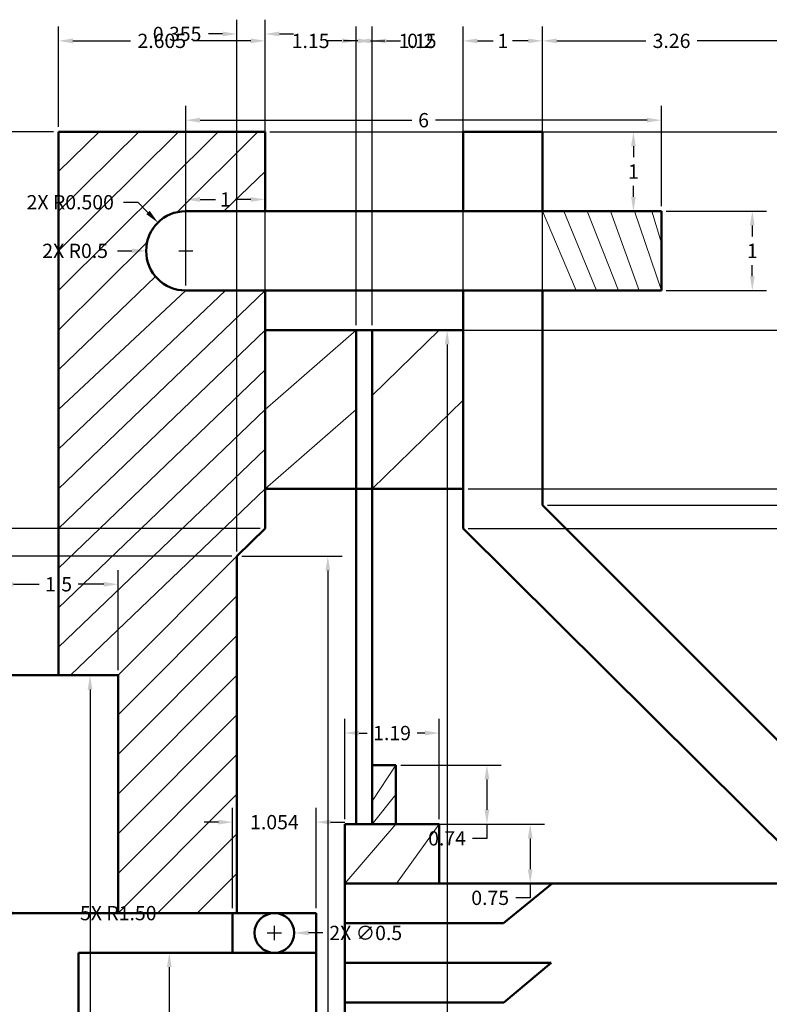
# Model space of a CAD drawing. Units: inches. Extents: x 15.4 to 41.1, y -0.4 to 25.1.
# Tile 3 of 4: x 20.3 to 29.7, y 12.7 to 25.1. Entities that reach past the tile are written whole.
import ezdxf

# ---------------------------------------------------------------- set-up
doc = ezdxf.new("R2010")
doc.units = ezdxf.units.IN
doc.header["$MEASUREMENT"] = 0
for name, color, linetype, lineweight in [('M-DIMS', 2, 'Continuous', 18), ('M-HATC', 8, 'Continuous', 18), ('M-OUTL', 7, 'Continuous', 50)]:
    doc.layers.add(name, color=color, linetype=linetype, lineweight=lineweight)
doc.styles.get("Standard").update_dxf_attribs({"font": 'arial.ttf'})
doc.dimstyles.get("Standard").update_dxf_attribs({"dimtxt": 0.18, "dimasz": 0.18, "dimexe": 0.18, "dimexo": 0.0625, "dimgap": 0.09, "dimtad": 0, "dimtih": 1, "dimtoh": 1, "dimdec": 4, "dimzin": 0, "dimdsep": 46, "dimtxsty": 'Standard', "dimcen": 0.09, "dimadec": 0, "dimazin": 0, "dimtfac": 1, "dimtdec": 4, "dimtofl": 0, "dimtmove": 0, "dimatfit": 3, "dimfxl": 1, "dimtolj": 1, "dimtzin": 0, "dimarcsym": 0})

# ---------------------------------------------------------------- blocks, each defined once
blk = doc.blocks.new('*D2')
at = {"layer": 'Defpoints', "color": 0, "transparency": 16777216}
for p in [(16.366, 23.727), (20.763, 23.727), (20.763, 1.022)]:
    blk.add_point(p, dxfattribs=at)
at = {"layer": 'M-DIMS', "color": 0, "lineweight": -2, "transparency": 16777216}
for p, q in [((20.7, 23.727), (16.186, 23.727)), ((16.366, 23.547), (16.366, 12.557)), ((16.366, 1.202), (16.366, 12.193)), ((20.7, 1.022), (16.186, 1.022))]:
    blk.add_line(p, q, dxfattribs=at)
at = {"layer": 'M-DIMS', "color": 0, "transparency": 16777216}
for points in [[(16.336, 23.547), (16.396, 23.547), (16.366, 23.727)], [(16.336, 1.202), (16.396, 1.202), (16.366, 1.022)]]:
    blk.add_solid(points, dxfattribs=at)
at = {"layer": 'M-DIMS', "color": 0, "transparency": 16777216, "insert": (16.366, 12.375), "char_height": 0.18, "attachment_point": 5}
blk.add_mtext('\\A1;22.705', dxfattribs=at)
blk = doc.blocks.new('*D3')
at = {"layer": 'Defpoints', "color": 0, "transparency": 16777216}
for p in [(23.368, 24.875), (20.763, 23.727), (23.368, 23.727)]:
    blk.add_point(p, dxfattribs=at)
at = {"layer": 'M-DIMS', "color": 0, "lineweight": -2, "transparency": 16777216}
for p, q in [((20.763, 23.79), (20.763, 25.055)), ((23.368, 23.79), (23.368, 25.055)), ((20.943, 24.875), (21.669, 24.875)), ((23.188, 24.875), (22.461, 24.875))]:
    blk.add_line(p, q, dxfattribs=at)
at = {"layer": 'M-DIMS', "color": 0, "transparency": 16777216}
for points in [[(20.943, 24.905), (20.943, 24.845), (20.763, 24.875)], [(23.188, 24.905), (23.188, 24.845), (23.368, 24.875)]]:
    blk.add_solid(points, dxfattribs=at)
at = {"layer": 'M-DIMS', "color": 0, "transparency": 16777216, "insert": (22.065, 24.875), "char_height": 0.18, "attachment_point": 5}
blk.add_mtext('\\A1;2.605', dxfattribs=at)
blk = doc.blocks.new('*D4')
at = {"layer": 'Defpoints', "color": 0, "transparency": 16777216}
for p in [(24.51758, 24.874511), (23.36758, 21.227011), (24.51758, 21.227011)]:
    blk.add_point(p, dxfattribs=at)
at = {"layer": 'M-DIMS', "color": 0, "lineweight": -2, "transparency": 16777216}
for p, q in [((23.36758, 21.289511), (23.36758, 25.054511)), ((24.51758, 21.289511), (24.51758, 25.054511)), ((23.18758, 24.874511), (23.00758, 24.874511)), ((24.69758, 24.874511), (24.87758, 24.874511))]:
    blk.add_line(p, q, dxfattribs=at)
at = {"layer": 'M-DIMS', "color": 0, "transparency": 16777216}
for points in [[(23.18758, 24.904511), (23.18758, 24.844511), (23.36758, 24.874511)], [(24.69758, 24.904511), (24.69758, 24.844511), (24.51758, 24.874511)]]:
    blk.add_solid(points, dxfattribs=at)
at = {"layer": 'M-DIMS', "color": 0, "transparency": 16777216, "insert": (23.94258, 24.874511), "char_height": 0.18, "attachment_point": 5}
blk.add_mtext('\\A1;1.15', dxfattribs=at)
blk = doc.blocks.new('*D5')
at = {"layer": 'Defpoints', "color": 0, "transparency": 16777216}
for p in [(24.718, 24.875), (24.518, 21.227), (24.718, 21.227)]:
    blk.add_point(p, dxfattribs=at)
at = {"layer": 'M-DIMS', "color": 0, "lineweight": -2, "transparency": 16777216}
for p, q in [((24.518, 21.29), (24.518, 25.055)), ((24.718, 21.29), (24.718, 25.055)), ((24.338, 24.875), (24.158, 24.875)), ((24.898, 24.875), (25.078, 24.875))]:
    blk.add_line(p, q, dxfattribs=at)
at = {"layer": 'M-DIMS', "color": 0, "transparency": 16777216}
for points in [[(24.338, 24.905), (24.338, 24.845), (24.518, 24.875)], [(24.898, 24.905), (24.898, 24.845), (24.718, 24.875)]]:
    blk.add_solid(points, dxfattribs=at)
at = {"layer": 'M-DIMS', "color": 0, "transparency": 16777216, "insert": (25.331, 24.875), "char_height": 0.18, "attachment_point": 5}
blk.add_mtext('\\A1;0.2', dxfattribs=at)
blk = doc.blocks.new('*D6')
at = {"layer": 'Defpoints', "color": 0, "transparency": 16777216}
for p in [(25.86758, 24.874511), (24.71758, 21.227011), (25.86758, 21.227011)]:
    blk.add_point(p, dxfattribs=at)
at = {"layer": 'M-DIMS', "color": 0, "lineweight": -2, "transparency": 16777216}
for p, q in [((24.71758, 21.289511), (24.71758, 25.054511)), ((25.86758, 21.289511), (25.86758, 25.054511)), ((24.53758, 24.874511), (24.35758, 24.874511)), ((26.04758, 24.874511), (26.22758, 24.874511))]:
    blk.add_line(p, q, dxfattribs=at)
at = {"layer": 'M-DIMS', "color": 0, "transparency": 16777216}
for points in [[(24.53758, 24.904511), (24.53758, 24.844511), (24.71758, 24.874511)], [(26.04758, 24.904511), (26.04758, 24.844511), (25.86758, 24.874511)]]:
    blk.add_solid(points, dxfattribs=at)
at = {"layer": 'M-DIMS', "color": 0, "transparency": 16777216, "insert": (25.29258, 24.874511), "char_height": 0.18, "attachment_point": 5}
blk.add_mtext('\\A1;1.15', dxfattribs=at)
blk = doc.blocks.new('*D7')
at = {"layer": 'Defpoints', "color": 0, "transparency": 16777216}
for p in [(26.868, 24.875), (25.868, 23.727), (26.868, 23.727)]:
    blk.add_point(p, dxfattribs=at)
at = {"layer": 'M-DIMS', "color": 0, "lineweight": -2, "transparency": 16777216}
for p, q in [((25.868, 23.79), (25.868, 25.055)), ((26.868, 23.79), (26.868, 25.055)), ((26.048, 24.875), (26.244, 24.875)), ((26.688, 24.875), (26.491, 24.875))]:
    blk.add_line(p, q, dxfattribs=at)
at = {"layer": 'M-DIMS', "color": 0, "transparency": 16777216}
for points in [[(26.048, 24.905), (26.048, 24.845), (25.868, 24.875)], [(26.688, 24.905), (26.688, 24.845), (26.868, 24.875)]]:
    blk.add_solid(points, dxfattribs=at)
at = {"layer": 'M-DIMS', "color": 0, "transparency": 16777216, "insert": (26.368, 24.875), "char_height": 0.18, "attachment_point": 5}
blk.add_mtext('\\A1;1', dxfattribs=at)
blk = doc.blocks.new('*D8')
at = {"layer": 'Defpoints', "color": 0, "transparency": 16777216}
for p in [(30.124, 24.875), (26.868, 19.021), (30.124, 14.498)]:
    blk.add_point(p, dxfattribs=at)
at = {"layer": 'M-DIMS', "color": 0, "lineweight": -2, "transparency": 16777216}
for p, q in [((26.868, 19.083), (26.868, 25.055)), ((30.124, 14.561), (30.124, 25.055)), ((27.048, 24.875), (28.172, 24.875)), ((29.944, 24.875), (28.819, 24.875))]:
    blk.add_line(p, q, dxfattribs=at)
at = {"layer": 'M-DIMS', "color": 0, "transparency": 16777216}
for points in [[(27.048, 24.905), (27.048, 24.845), (26.868, 24.875)], [(29.944, 24.905), (29.944, 24.845), (30.124, 24.875)]]:
    blk.add_solid(points, dxfattribs=at)
at = {"layer": 'M-DIMS', "color": 0, "transparency": 16777216, "insert": (28.496, 24.875), "char_height": 0.18, "attachment_point": 5}
blk.add_mtext('\\A1;3.26', dxfattribs=at)
blk = doc.blocks.new('*D11')
at = {"layer": 'Defpoints', "color": 0, "transparency": 16777216}
for p in [(26.868, 23.727), (25.868, 18.727), (40.699, 18.727)]:
    blk.add_point(p, dxfattribs=at)
at = {"layer": 'M-DIMS', "color": 0, "lineweight": -2, "transparency": 16777216}
for p, q in [((26.93, 23.727), (40.879, 23.727)), ((40.699, 23.547), (40.699, 21.409)), ((40.699, 18.907), (40.699, 21.045)), ((25.93, 18.727), (40.879, 18.727))]:
    blk.add_line(p, q, dxfattribs=at)
at = {"layer": 'M-DIMS', "color": 0, "transparency": 16777216}
for points in [[(40.669, 23.547), (40.729, 23.547), (40.699, 23.727)], [(40.669, 18.907), (40.729, 18.907), (40.699, 18.727)]]:
    blk.add_solid(points, dxfattribs=at)
at = {"layer": 'M-DIMS', "color": 0, "transparency": 16777216, "insert": (40.699, 21.227), "char_height": 0.18, "attachment_point": 5}
blk.add_mtext('\\A1;5', dxfattribs=at)
blk = doc.blocks.new('*D12')
at = {"layer": 'Defpoints', "color": 0, "transparency": 16777216}
for p in [(25.868, 18.727), (30.124, 14.498), (40.699, 14.498)]:
    blk.add_point(p, dxfattribs=at)
at = {"layer": 'M-DIMS', "color": 0, "lineweight": -2, "transparency": 16777216}
for p, q in [((25.93, 18.727), (40.879, 18.727)), ((40.699, 18.547), (40.699, 16.794)), ((40.699, 14.678), (40.699, 16.431)), ((30.186, 14.498), (40.879, 14.498))]:
    blk.add_line(p, q, dxfattribs=at)
at = {"layer": 'M-DIMS', "color": 0, "transparency": 16777216}
for points in [[(40.669, 18.547), (40.729, 18.547), (40.699, 18.727)], [(40.669, 14.678), (40.729, 14.678), (40.699, 14.498)]]:
    blk.add_solid(points, dxfattribs=at)
at = {"layer": 'M-DIMS', "color": 0, "transparency": 16777216, "insert": (40.699, 16.613), "char_height": 0.18, "attachment_point": 5}
blk.add_mtext('\\A1;4.229', dxfattribs=at)
blk = doc.blocks.new('*D13')
at = {"layer": 'Defpoints', "color": 0, "transparency": 16777216}
for p in [(28.368, 23.875), (22.368, 22.727), (28.368, 22.727)]:
    blk.add_point(p, dxfattribs=at)
at = {"layer": 'M-DIMS', "color": 0, "lineweight": -2, "transparency": 16777216}
for p, q in [((22.368, 22.79), (22.368, 24.055)), ((28.368, 22.79), (28.368, 24.055)), ((22.548, 23.875), (25.218, 23.875)), ((28.188, 23.875), (25.517, 23.875))]:
    blk.add_line(p, q, dxfattribs=at)
at = {"layer": 'M-DIMS', "color": 0, "transparency": 16777216}
for points in [[(22.548, 23.905), (22.548, 23.845), (22.368, 23.875)], [(28.188, 23.905), (28.188, 23.845), (28.368, 23.875)]]:
    blk.add_solid(points, dxfattribs=at)
at = {"layer": 'M-DIMS', "color": 0, "transparency": 16777216, "insert": (25.368, 23.875), "char_height": 0.18, "attachment_point": 5}
blk.add_mtext('\\A1;6', dxfattribs=at)
blk = doc.blocks.new('*D14')
at = {"layer": 'Defpoints', "color": 0, "transparency": 16777216}
for p in [(28.368, 22.727), (28.368, 21.727), (29.515, 21.727)]:
    blk.add_point(p, dxfattribs=at)
at = {"layer": 'M-DIMS', "color": 0, "lineweight": -2, "transparency": 16777216}
for p, q in [((28.43, 22.727), (29.695, 22.727)), ((29.515, 22.547), (29.515, 22.407)), ((29.515, 21.907), (29.515, 22.047)), ((28.43, 21.727), (29.695, 21.727))]:
    blk.add_line(p, q, dxfattribs=at)
at = {"layer": 'M-DIMS', "color": 0, "transparency": 16777216}
for points in [[(29.485, 22.547), (29.545, 22.547), (29.515, 22.727)], [(29.485, 21.907), (29.545, 21.907), (29.515, 21.727)]]:
    blk.add_solid(points, dxfattribs=at)
at = {"layer": 'M-DIMS', "color": 0, "transparency": 16777216, "insert": (29.515, 22.227), "char_height": 0.18, "attachment_point": 5}
blk.add_mtext('\\A1;1', dxfattribs=at)
blk = doc.blocks.new('*D15')
at = {"layer": 'Defpoints', "color": 0, "transparency": 16777216}
for p in [(26.868, 23.727), (26.868, 22.727), (28.015, 22.727)]:
    blk.add_point(p, dxfattribs=at)
at = {"layer": 'M-DIMS', "color": 0, "lineweight": -2, "transparency": 16777216}
for p, q in [((26.93, 23.727), (28.195, 23.727)), ((28.015, 23.547), (28.015, 23.407)), ((28.015, 22.907), (28.015, 23.047)), ((26.93, 22.727), (28.195, 22.727))]:
    blk.add_line(p, q, dxfattribs=at)
at = {"layer": 'M-DIMS', "color": 0, "transparency": 16777216}
for points in [[(27.985, 23.547), (28.045, 23.547), (28.015, 23.727)], [(27.985, 22.907), (28.045, 22.907), (28.015, 22.727)]]:
    blk.add_solid(points, dxfattribs=at)
at = {"layer": 'M-DIMS', "color": 0, "transparency": 16777216, "insert": (28.015, 23.227), "char_height": 0.18, "attachment_point": 5}
blk.add_mtext('\\A1;1', dxfattribs=at)
blk = doc.blocks.new('*D16')
at = {"layer": 'Defpoints', "color": 0, "transparency": 16777216}
for p in [(23.368, 22.875), (22.368, 21.727), (23.368, 21.727)]:
    blk.add_point(p, dxfattribs=at)
at = {"layer": 'M-DIMS', "color": 0, "lineweight": -2, "transparency": 16777216}
for p, q in [((22.368, 21.79), (22.368, 23.055)), ((23.368, 21.79), (23.368, 23.055)), ((22.548, 22.875), (22.744, 22.875)), ((23.188, 22.875), (22.991, 22.875))]:
    blk.add_line(p, q, dxfattribs=at)
at = {"layer": 'M-DIMS', "color": 0, "transparency": 16777216}
for points in [[(22.548, 22.905), (22.548, 22.845), (22.368, 22.875)], [(23.188, 22.905), (23.188, 22.845), (23.368, 22.875)]]:
    blk.add_solid(points, dxfattribs=at)
at = {"layer": 'M-DIMS', "color": 0, "transparency": 16777216, "insert": (22.868, 22.875), "char_height": 0.18, "attachment_point": 5}
blk.add_mtext('\\A1;1', dxfattribs=at)
blk = doc.blocks.new('*D18')
at = {"layer": 'Defpoints', "color": 0, "transparency": 16777216}
for p in [(24.518, 21.227), (24.518, 3.522), (25.665, 3.522)]:
    blk.add_point(p, dxfattribs=at)
at = {"layer": 'M-DIMS', "color": 0, "lineweight": -2, "transparency": 16777216}
for p, q in [((24.58, 21.227), (25.845, 21.227)), ((25.665, 21.047), (25.665, 12.557)), ((25.665, 3.702), (25.665, 12.193)), ((24.58, 3.522), (25.845, 3.522))]:
    blk.add_line(p, q, dxfattribs=at)
at = {"layer": 'M-DIMS', "color": 0, "transparency": 16777216}
for points in [[(25.635, 21.047), (25.695, 21.047), (25.665, 21.227)], [(25.635, 3.702), (25.695, 3.702), (25.665, 3.522)]]:
    blk.add_solid(points, dxfattribs=at)
at = {"layer": 'M-DIMS', "color": 0, "transparency": 16777216, "insert": (25.665, 12.375), "char_height": 0.18, "attachment_point": 5}
blk.add_mtext('\\A1;17.705', dxfattribs=at)
blk = doc.blocks.new('*D19')
at = {"layer": 'Defpoints', "color": 0, "transparency": 16777216}
for p in [(23.013, 18.375), (23.013, 6.375), (24.16, 6.375)]:
    blk.add_point(p, dxfattribs=at)
at = {"layer": 'M-DIMS', "color": 0, "lineweight": -2, "transparency": 16777216}
for p, q in [((23.075, 18.375), (24.34, 18.375)), ((24.16, 18.195), (24.16, 12.555)), ((24.16, 6.555), (24.16, 12.194)), ((23.075, 6.375), (24.34, 6.375))]:
    blk.add_line(p, q, dxfattribs=at)
at = {"layer": 'M-DIMS', "color": 0, "transparency": 16777216}
for points in [[(24.13, 18.195), (24.19, 18.195), (24.16, 18.375)], [(24.13, 6.555), (24.19, 6.555), (24.16, 6.375)]]:
    blk.add_solid(points, dxfattribs=at)
at = {"layer": 'M-DIMS', "color": 0, "transparency": 16777216, "insert": (24.16, 12.375), "char_height": 0.18, "attachment_point": 5}
blk.add_mtext('\\A1;12', dxfattribs=at)
blk = doc.blocks.new('*D20')
at = {"layer": 'Defpoints', "color": 0, "transparency": 16777216}
for p in [(21.513, 18.022), (20.013, 16.875), (21.513, 16.875)]:
    blk.add_point(p, dxfattribs=at)
at = {"layer": 'M-DIMS', "color": 0, "lineweight": -2, "transparency": 16777216}
for p, q in [((20.013, 16.937), (20.013, 18.202)), ((21.513, 16.937), (21.513, 18.202)), ((20.193, 18.022), (20.517, 18.022)), ((21.333, 18.022), (21.009, 18.022))]:
    blk.add_line(p, q, dxfattribs=at)
at = {"layer": 'M-DIMS', "color": 0, "transparency": 16777216}
for points in [[(20.193, 18.052), (20.193, 17.992), (20.013, 18.022)], [(21.333, 18.052), (21.333, 17.992), (21.513, 18.022)]]:
    blk.add_solid(points, dxfattribs=at)
at = {"layer": 'M-DIMS', "color": 0, "transparency": 16777216, "insert": (20.763, 18.022), "char_height": 0.18, "attachment_point": 5}
blk.add_mtext('\\A1;1.5', dxfattribs=at)
blk = doc.blocks.new('*D21')
at = {"layer": 'Defpoints', "color": 0, "transparency": 16777216}
for p in [(20.013, 16.875), (20.013, 7.875), (21.16, 7.875)]:
    blk.add_point(p, dxfattribs=at)
at = {"layer": 'M-DIMS', "color": 0, "lineweight": -2, "transparency": 16777216}
for p, q in [((20.075, 16.875), (21.34, 16.875)), ((21.16, 16.695), (21.16, 12.557)), ((21.16, 8.055), (21.16, 12.193)), ((20.075, 7.875), (21.34, 7.875))]:
    blk.add_line(p, q, dxfattribs=at)
at = {"layer": 'M-DIMS', "color": 0, "transparency": 16777216}
for points in [[(21.13, 16.695), (21.19, 16.695), (21.16, 16.875)], [(21.13, 8.055), (21.19, 8.055), (21.16, 7.875)]]:
    blk.add_solid(points, dxfattribs=at)
at = {"layer": 'M-DIMS', "color": 0, "transparency": 16777216, "insert": (21.16, 12.375), "char_height": 0.18, "attachment_point": 5}
blk.add_mtext('\\A1;9', dxfattribs=at)
blk = doc.blocks.new('*D24')
at = {"layer": 'Defpoints', "color": 0, "transparency": 16777216}
for p in [(21.013, 13.375), (21.013, 11.375), (22.16, 11.375)]:
    blk.add_point(p, dxfattribs=at)
at = {"layer": 'M-DIMS', "color": 0, "lineweight": -2, "transparency": 16777216}
for p, q in [((21.075, 13.375), (22.34, 13.375)), ((22.16, 13.195), (22.16, 12.555)), ((22.16, 11.555), (22.16, 12.194)), ((21.075, 11.375), (22.34, 11.375))]:
    blk.add_line(p, q, dxfattribs=at)
at = {"layer": 'M-DIMS', "color": 0, "transparency": 16777216}
for points in [[(22.13, 13.195), (22.19, 13.195), (22.16, 13.375)], [(22.13, 11.555), (22.19, 11.555), (22.16, 11.375)]]:
    blk.add_solid(points, dxfattribs=at)
at = {"layer": 'M-DIMS', "color": 0, "transparency": 16777216, "insert": (22.16, 12.375), "char_height": 0.18, "attachment_point": 5}
blk.add_mtext('\\A1;2', dxfattribs=at)
blk = doc.blocks.new('*D26')
at = {"layer": 'Defpoints', "color": 0, "transparency": 16777216}
for p in [(24.012794, 15.022195), (22.958846, 13.874695), (24.012794, 13.874695)]:
    blk.add_point(p, dxfattribs=at)
at = {"layer": 'M-DIMS', "color": 0, "lineweight": -2, "transparency": 16777216}
for p, q in [((22.958846, 13.937195), (22.958846, 15.202195)), ((24.012794, 13.937195), (24.012794, 15.202195)), ((22.778846, 15.022195), (22.598846, 15.022195)), ((24.192794, 15.022195), (24.372794, 15.022195))]:
    blk.add_line(p, q, dxfattribs=at)
at = {"layer": 'M-DIMS', "color": 0, "transparency": 16777216}
for points in [[(22.778846, 15.052195), (22.778846, 14.992195), (22.958846, 15.022195)], [(24.192794, 15.052195), (24.192794, 14.992195), (24.012794, 15.022195)]]:
    blk.add_solid(points, dxfattribs=at)
at = {"layer": 'M-DIMS', "color": 0, "transparency": 16777216, "insert": (23.48582, 15.022195), "char_height": 0.18, "attachment_point": 5}
blk.add_mtext('\\A1;1.054', dxfattribs=at)
blk = doc.blocks.new('*D27')
at = {"layer": 'Defpoints', "color": 0, "transparency": 16777216}
for p in [(25.565, 16.146), (24.374, 14.998), (25.565, 14.998)]:
    blk.add_point(p, dxfattribs=at)
at = {"layer": 'M-DIMS', "color": 0, "lineweight": -2, "transparency": 16777216}
for p, q in [((24.374, 15.061), (24.374, 16.326)), ((25.565, 15.061), (25.565, 16.326)), ((24.554, 16.146), (24.654, 16.146)), ((25.385, 16.146), (25.285, 16.146))]:
    blk.add_line(p, q, dxfattribs=at)
at = {"layer": 'M-DIMS', "color": 0, "transparency": 16777216}
for points in [[(24.554, 16.176), (24.554, 16.116), (24.374, 16.146)], [(25.385, 16.176), (25.385, 16.116), (25.565, 16.146)]]:
    blk.add_solid(points, dxfattribs=at)
at = {"layer": 'M-DIMS', "color": 0, "transparency": 16777216, "insert": (24.97, 16.146), "char_height": 0.18, "attachment_point": 5}
blk.add_mtext('\\A1;1.19', dxfattribs=at)
blk = doc.blocks.new('*D28')
at = {"layer": 'Defpoints', "color": 0, "transparency": 16777216}
for p in [(25.565, 14.998), (25.565, 14.248), (26.713, 14.248)]:
    blk.add_point(p, dxfattribs=at)
at = {"layer": 'M-DIMS', "color": 0, "lineweight": -2, "transparency": 16777216}
for p, q in [((25.628, 14.998), (26.893, 14.998)), ((26.713, 14.818), (26.713, 14.428)), ((25.628, 14.248), (26.893, 14.248)), ((26.713, 14.248), (26.713, 14.068)), ((26.713, 14.068), (26.533, 14.068))]:
    blk.add_line(p, q, dxfattribs=at)
at = {"layer": 'M-DIMS', "color": 0, "transparency": 16777216}
for points in [[(26.683, 14.818), (26.743, 14.818), (26.713, 14.998)], [(26.683, 14.428), (26.743, 14.428), (26.713, 14.248)]]:
    blk.add_solid(points, dxfattribs=at)
at = {"layer": 'M-DIMS', "color": 0, "transparency": 16777216, "insert": (26.208, 14.068), "char_height": 0.18, "attachment_point": 5}
blk.add_mtext('\\A1;0.75', dxfattribs=at)
blk = doc.blocks.new('*D29')
at = {"layer": 'Defpoints', "color": 0, "transparency": 16777216}
for p in [(25.02, 15.742), (25.02, 14.998), (26.167, 14.998)]:
    blk.add_point(p, dxfattribs=at)
at = {"layer": 'M-DIMS', "color": 0, "lineweight": -2, "transparency": 16777216}
for p, q in [((25.082, 15.742), (26.347, 15.742)), ((26.167, 15.562), (26.167, 15.178)), ((25.082, 14.998), (26.347, 14.998)), ((26.167, 14.998), (26.167, 14.818)), ((26.167, 14.818), (25.987, 14.818))]:
    blk.add_line(p, q, dxfattribs=at)
at = {"layer": 'M-DIMS', "color": 0, "transparency": 16777216}
for points in [[(26.137, 15.562), (26.197, 15.562), (26.167, 15.742)], [(26.137, 15.178), (26.197, 15.178), (26.167, 14.998)]]:
    blk.add_solid(points, dxfattribs=at)
at = {"layer": 'M-DIMS', "color": 0, "transparency": 16777216, "insert": (25.664, 14.818), "char_height": 0.18, "attachment_point": 5}
blk.add_mtext('\\A1;0.74', dxfattribs=at)
blk = doc.blocks.new('*D35')
at = {"layer": 'Defpoints', "color": 0, "transparency": 16777216}
for p in [(18.513, 13.875), (20.013, 13.875)]:
    blk.add_point(p, dxfattribs=at)
at = {"layer": 'M-DIMS', "color": 0, "lineweight": -2, "transparency": 16777216}
for p, q in [((18.513, 13.785), (18.513, 13.965)), ((18.423, 13.875), (18.603, 13.875)), ((20.913, 13.875), (20.193, 13.875))]:
    blk.add_line(p, q, dxfattribs=at)
at = {"layer": 'M-DIMS', "color": 0, "transparency": 16777216}
blk.add_solid([(20.193, 13.905), (20.193, 13.845), (20.013, 13.875)], dxfattribs=at)
at = {"layer": 'M-DIMS', "color": 0, "transparency": 16777216, "insert": (21.516, 13.875), "char_height": 0.18, "attachment_point": 5}
blk.add_mtext('\\A1;5X R1.50', dxfattribs=at)
blk = doc.blocks.new('*D37')
at = {"layer": 'Defpoints', "color": 0, "transparency": 16777216}
for p in [(21.868, 22.227), (22.368, 22.227)]:
    blk.add_point(p, dxfattribs=at)
at = {"layer": 'M-DIMS', "color": 0, "lineweight": -2, "transparency": 16777216}
for p, q in [((21.508, 22.227), (21.688, 22.227)), ((22.278, 22.227), (22.458, 22.227)), ((22.368, 22.137), (22.368, 22.317))]:
    blk.add_line(p, q, dxfattribs=at)
at = {"layer": 'M-DIMS', "color": 0, "transparency": 16777216}
blk.add_solid([(21.688, 22.257), (21.688, 22.197), (21.868, 22.227)], dxfattribs=at)
at = {"layer": 'M-DIMS', "color": 0, "transparency": 16777216, "insert": (20.972, 22.227), "char_height": 0.18, "attachment_point": 5}
blk.add_mtext('\\A1;2X R0.5', dxfattribs=at)
blk = doc.blocks.new('*D40')
at = {"layer": 'Defpoints', "color": 0, "transparency": 16777216}
for p in [(23.236, 13.624), (23.736, 13.625)]:
    blk.add_point(p, dxfattribs=at)
at = {"layer": 'M-DIMS', "color": 0, "lineweight": -2, "transparency": 16777216}
for p, q in [((23.486, 13.535), (23.486, 13.715)), ((23.396, 13.625), (23.576, 13.625)), ((24.096, 13.625), (23.916, 13.625))]:
    blk.add_line(p, q, dxfattribs=at)
at = {"layer": 'M-DIMS', "color": 0, "transparency": 16777216}
blk.add_solid([(23.916, 13.655), (23.916, 13.595), (23.736, 13.625)], dxfattribs=at)
at = {"layer": 'M-DIMS', "color": 0, "transparency": 16777216, "insert": (24.638, 13.625), "char_height": 0.18, "attachment_point": 5}
blk.add_mtext('\\A1;2X ∅0.5', dxfattribs=at)
blk = doc.blocks.new('*D41')
at = {"layer": 'Defpoints', "color": 0, "transparency": 16777216}
for p in [(23.013, 24.962), (23.368, 18.727), (23.013, 18.375)]:
    blk.add_point(p, dxfattribs=at)
at = {"layer": 'M-DIMS', "color": 0, "lineweight": -2, "transparency": 16777216}
for p, q in [((23.013, 18.437), (23.013, 25.142)), ((23.368, 18.79), (23.368, 25.142)), ((22.833, 24.962), (22.653, 24.962)), ((23.548, 24.962), (23.728, 24.962))]:
    blk.add_line(p, q, dxfattribs=at)
at = {"layer": 'M-DIMS', "color": 0, "transparency": 16777216}
for points in [[(22.833, 24.992), (22.833, 24.932), (23.013, 24.962)], [(23.548, 24.992), (23.548, 24.932), (23.368, 24.962)]]:
    blk.add_solid(points, dxfattribs=at)
at = {"layer": 'M-DIMS', "color": 0, "transparency": 16777216, "insert": (22.258, 24.962), "char_height": 0.18, "attachment_point": 5}
blk.add_mtext('\\A1;0.355', dxfattribs=at)
blk = doc.blocks.new('*D42')
at = {"layer": 'Defpoints', "color": 0, "transparency": 16777216}
for p in [(23.368, 18.727), (16.278, 18.375), (23.013, 18.375)]:
    blk.add_point(p, dxfattribs=at)
at = {"layer": 'M-DIMS', "color": 0, "lineweight": -2, "transparency": 16777216}
for p, q in [((16.278, 18.907), (16.278, 19.087)), ((23.305, 18.727), (16.098, 18.727)), ((22.95, 18.375), (16.098, 18.375)), ((16.278, 18.195), (16.278, 18.015)), ((16.278, 18.015), (16.098, 18.015))]:
    blk.add_line(p, q, dxfattribs=at)
at = {"layer": 'M-DIMS', "color": 0, "transparency": 16777216}
for points in [[(16.248, 18.907), (16.308, 18.907), (16.278, 18.727)], [(16.248, 18.195), (16.308, 18.195), (16.278, 18.375)]]:
    blk.add_solid(points, dxfattribs=at)
at = {"layer": 'M-DIMS', "color": 0, "transparency": 16777216, "insert": (15.705, 18.015), "char_height": 0.18, "attachment_point": 5}
blk.add_mtext('\\A1;0.352', dxfattribs=at)
blk = doc.blocks.new('*D43')
at = {"layer": 'Defpoints', "color": 0, "transparency": 16777216}
for p in [(23.368, 23.727), (23.368, 21.227), (40.787, 21.227)]:
    blk.add_point(p, dxfattribs=at)
at = {"layer": 'M-DIMS', "color": 0, "lineweight": -2, "transparency": 16777216}
for p, q in [((23.43, 23.727), (40.967, 23.727)), ((40.787, 23.547), (40.787, 22.659)), ((40.787, 21.407), (40.787, 22.295)), ((23.43, 21.227), (40.967, 21.227))]:
    blk.add_line(p, q, dxfattribs=at)
at = {"layer": 'M-DIMS', "color": 0, "transparency": 16777216}
for points in [[(40.757, 23.547), (40.817, 23.547), (40.787, 23.727)], [(40.757, 21.407), (40.817, 21.407), (40.787, 21.227)]]:
    blk.add_solid(points, dxfattribs=at)
at = {"layer": 'M-DIMS', "color": 0, "transparency": 16777216, "insert": (40.787, 22.477), "char_height": 0.18, "attachment_point": 5}
blk.add_mtext('\\A1;2.500', dxfattribs=at)
blk = doc.blocks.new('*D44')
at = {"layer": 'Defpoints', "color": 0, "transparency": 16777216}
for p in [(25.868, 21.227), (25.868, 19.227), (40.787, 19.227)]:
    blk.add_point(p, dxfattribs=at)
at = {"layer": 'M-DIMS', "color": 0, "lineweight": -2, "transparency": 16777216}
for p, q in [((25.93, 21.227), (40.967, 21.227)), ((40.787, 21.047), (40.787, 20.409)), ((40.787, 19.407), (40.787, 20.045)), ((25.93, 19.227), (40.967, 19.227))]:
    blk.add_line(p, q, dxfattribs=at)
at = {"layer": 'M-DIMS', "color": 0, "transparency": 16777216}
for points in [[(40.757, 21.047), (40.817, 21.047), (40.787, 21.227)], [(40.757, 19.407), (40.817, 19.407), (40.787, 19.227)]]:
    blk.add_solid(points, dxfattribs=at)
at = {"layer": 'M-DIMS', "color": 0, "transparency": 16777216, "insert": (40.787, 20.227), "char_height": 0.18, "attachment_point": 5}
blk.add_mtext('\\A1;2.000', dxfattribs=at)
blk = doc.blocks.new('*D46')
at = {"layer": 'Defpoints', "color": 0, "transparency": 16777216}
for p in [(26.868, 23.727), (26.868, 19.021), (40.787, 19.021)]:
    blk.add_point(p, dxfattribs=at)
at = {"layer": 'M-DIMS', "color": 0, "lineweight": -2, "transparency": 16777216}
for p, q in [((26.93, 23.727), (40.967, 23.727)), ((40.787, 23.547), (40.787, 21.556)), ((40.787, 19.201), (40.787, 21.192)), ((26.93, 19.021), (40.967, 19.021))]:
    blk.add_line(p, q, dxfattribs=at)
at = {"layer": 'M-DIMS', "color": 0, "transparency": 16777216}
for points in [[(40.757, 23.547), (40.817, 23.547), (40.787, 23.727)], [(40.757, 19.201), (40.817, 19.201), (40.787, 19.021)]]:
    blk.add_solid(points, dxfattribs=at)
at = {"layer": 'M-DIMS', "color": 0, "transparency": 16777216, "insert": (40.787, 21.374), "char_height": 0.18, "attachment_point": 5}
blk.add_mtext('\\A1;4.706', dxfattribs=at)
blk = doc.blocks.new('*D57')
at = {"layer": 'Defpoints', "color": 0, "transparency": 16777216}
for p in [(22.017, 22.583), (22.368, 22.227)]:
    blk.add_point(p, dxfattribs=at)
at = {"layer": 'M-DIMS', "color": 0, "lineweight": -2, "transparency": 16777216}
for p, q in [((21.584, 22.84), (21.764, 22.84)), ((21.764, 22.84), (21.89, 22.712)), ((22.278, 22.227), (22.458, 22.227)), ((22.368, 22.137), (22.368, 22.317))]:
    blk.add_line(p, q, dxfattribs=at)
at = {"layer": 'M-DIMS', "color": 0, "transparency": 16777216}
blk.add_solid([(21.912, 22.733), (21.869, 22.69), (22.017, 22.583)], dxfattribs=at)
at = {"layer": 'M-DIMS', "color": 0, "transparency": 16777216, "insert": (20.91, 22.84), "char_height": 0.18, "attachment_point": 5}
blk.add_mtext('\\A1;2X R0.500', dxfattribs=at)

msp = doc.modelspace()

# ---------------------------------------------------------------- linework, layer by layer
at = {"layer": 'M-HATC'}
for p, q in [((20.7628, 23.227), (21.2762, 23.727)), ((20.7628, 22.727), (21.7762, 23.727)), ((22.2762, 23.727), (20.7628, 22.227)), ((20.7628, 21.727), (22.7762, 23.727)), ((23.2762, 23.727), (22.2588, 22.715)), ((22.8466, 22.727), (23.3676, 23.227)), ((26.8676, 22.727), (27.2933, 21.727)), ((27.5483, 21.727), (27.1388, 22.727)), ((27.4324, 22.727), (27.8264, 21.727)), ((28.0892, 21.727), (27.726, 22.727)), ((28.0274, 22.727), (28.3676, 21.727)), ((28.2467, 22.727), (28.3676, 22.3252)), ((21.8801, 22.3384), (20.7628, 21.227)), ((20.7628, 20.727), (21.9874, 21.9023)), ((22.3676, 21.727), (20.7628, 20.227)), ((22.8676, 21.727), (20.7628, 19.727)), ((20.7628, 19.227), (23.3676, 21.727)), ((23.3676, 21.227), (20.7628, 18.727)), ((23.3676, 20.227), (24.5176, 21.227)), ((24.7176, 20.4009), (25.5644, 21.227)), ((20.7628, 18.227), (23.3676, 20.727)), ((24.7176, 19.227), (25.8676, 20.3453)), ((23.3676, 20.227), (20.7628, 17.727)), ((24.5176, 20.227), (23.3676, 19.227)), ((23.3676, 19.727), (20.7628, 17.227)), ((20.9128, 16.8747), (23.3676, 19.227)), ((23.0128, 18.3747), (21.5128, 16.8747)), ((21.5128, 16.3747), (23.0128, 17.8747)), ((23.0128, 17.3747), (21.5128, 15.8747)), ((21.5128, 15.3747), (23.0128, 16.8747)), ((23.0128, 16.3747), (21.5128, 14.8747)), ((21.5128, 14.3747), (23.0128, 15.8747)), ((25.0198, 15.7423), (24.7176, 15.2849)), ((23.0128, 15.3747), (21.5128, 13.8747)), ((24.7176, 14.9981), (25.0198, 15.3702)), ((24.374, 14.2482), (25.0198, 14.9981)), ((25.5651, 14.9981), (25.028, 14.2482)), ((22.0128, 13.8747), (23.0128, 14.8747)), ((22.5128, 13.8747), (23.0128, 14.3747))]:
    msp.add_line(p, q, dxfattribs=at)
at = {"layer": 'M-OUTL'}
for p, q in [((20.7628, 16.8747), (20.7628, 23.727)), ((23.3676, 23.727), (20.7628, 23.727)), ((20.7628, 23.727), (20.7628, 23.227)), ((21.2762, 23.727), (21.7762, 23.727)), ((21.7762, 23.727), (22.2762, 23.727)), ((21.7762, 23.727), (22.2762, 23.727)), ((22.2762, 23.727), (22.7762, 23.727)), ((22.7762, 23.727), (23.2762, 23.727)), ((22.7762, 23.727), (23.2762, 23.727)), ((23.3676, 22.727), (23.3676, 23.727)), ((23.3676, 23.727), (23.3676, 23.227)), ((25.8676, 22.727), (25.8676, 23.727)), ((25.8676, 23.727), (26.8676, 23.727)), ((26.8676, 23.727), (26.8676, 22.727)), ((20.7628, 23.227), (20.7628, 22.727)), ((20.7628, 22.727), (20.7628, 22.227)), ((22.3676, 22.727), (23.3676, 22.727)), ((23.3676, 22.727), (28.3676, 22.727)), ((27.1388, 22.727), (27.4324, 22.727)), ((27.726, 22.727), (28.0274, 22.727)), ((28.0274, 22.727), (28.2467, 22.727)), ((28.3676, 22.727), (28.3676, 21.727)), ((20.7628, 22.227), (20.7628, 21.727)), ((20.7628, 22.227), (20.7628, 21.727)), ((28.3676, 21.727), (28.3676, 22.3252)), ((20.7628, 21.727), (20.7628, 21.227)), ((23.3676, 21.727), (22.3676, 21.727)), ((22.3676, 21.727), (22.8676, 21.727)), ((23.3676, 18.727), (23.3676, 21.727)), ((28.3676, 21.727), (23.3676, 21.727)), ((23.3676, 21.727), (23.3676, 20.727)), ((23.3676, 21.727), (23.3676, 21.227)), ((23.3676, 21.727), (23.3676, 21.227)), ((25.8676, 21.727), (25.8676, 18.727)), ((26.8676, 21.727), (26.8676, 19.0206)), ((27.2933, 21.727), (27.5483, 21.727)), ((27.8264, 21.727), (28.0892, 21.727)), ((20.7628, 21.227), (20.7628, 20.727)), ((23.3676, 21.227), (25.8676, 21.227)), ((23.3676, 21.227), (24.5176, 21.227)), ((24.5176, 21.227), (24.5176, 19.227)), ((24.5176, 21.227), (24.5176, 20.227)), ((25.8676, 21.227), (24.7176, 21.227)), ((24.7176, 21.227), (24.7176, 15.5717)), ((20.7628, 20.727), (20.7628, 20.227)), ((23.3676, 20.727), (23.3676, 20.227)), ((20.7628, 20.227), (20.7628, 19.727)), ((23.3676, 20.227), (23.3676, 19.727)), ((20.7628, 19.727), (20.7628, 19.227)), ((20.7628, 19.227), (20.7628, 18.727)), ((23.3676, 18.727), (23.3676, 19.227)), ((23.3676, 19.227), (25.8676, 19.227)), ((24.5176, 19.227), (24.5176, 15.4836)), ((26.8676, 19.0206), (31.1089, 14.7766)), ((20.7628, 18.727), (20.7628, 18.227)), ((20.7628, 18.727), (20.7628, 18.227)), ((23.0128, 18.3747), (23.3676, 18.727)), ((25.8676, 18.727), (30.124, 14.4982)), ((23.0128, 17.8747), (23.0128, 18.3747)), ((23.0128, 18.3747), (23.0128, 17.8747)), ((20.7628, 18.227), (20.7628, 17.727)), ((23.0128, 13.8747), (23.0128, 17.8747)), ((23.0128, 17.8747), (23.0128, 17.3747)), ((23.0128, 17.8747), (23.0128, 17.3747)), ((20.7628, 17.727), (20.7628, 17.227)), ((20.7628, 17.727), (20.7628, 17.227)), ((23.0128, 17.3747), (23.0128, 16.8747)), ((20.7628, 17.227), (20.7628, 16.8747)), ((20.0128, 16.8747), (21.0128, 16.8747)), ((20.7628, 16.8747), (20.9128, 16.8747)), ((21.0128, 16.8747), (21.5128, 16.8747)), ((21.5128, 16.8747), (21.5128, 13.8747)), ((21.5128, 16.8747), (21.5128, 16.3747)), ((23.0128, 16.8747), (23.0128, 16.3747)), ((23.0128, 16.8747), (23.0128, 16.3747)), ((21.5128, 16.3747), (21.5128, 15.8747)), ((23.0128, 16.3747), (23.0128, 15.8747)), ((21.5128, 15.8747), (21.5128, 15.3747)), ((21.5128, 15.8747), (21.5128, 15.3747)), ((23.0128, 15.8747), (23.0128, 15.3747)), ((23.0128, 15.8747), (23.0128, 15.3747)), ((24.7176, 15.7423), (25.0198, 15.7423)), ((25.0198, 15.7423), (25.0198, 14.9981)), ((24.7176, 15.5717), (24.7176, 14.9981)), ((24.5176, 15.4836), (24.5176, 14.9981)), ((21.5128, 15.3747), (21.5128, 14.8747)), ((23.0128, 15.3747), (23.0128, 14.8747)), ((24.7176, 15.2849), (24.7176, 14.9981)), ((24.374, 14.2482), (24.374, 14.9981)), ((24.374, 14.9981), (25.5651, 14.9981)), ((25.0198, 14.9981), (25.5651, 14.9981)), ((25.5651, 14.9981), (25.5651, 14.2482)), ((21.5128, 14.8747), (21.5128, 14.3747)), ((21.5128, 14.8747), (21.5128, 14.3747)), ((23.0128, 14.8747), (23.0128, 14.3747)), ((24.374, 10.5012), (24.374, 14.5012)), ((24.374, 10.5012), (24.374, 14.5012)), ((21.5128, 14.3747), (21.5128, 13.8747)), ((30.124, 14.2482), (24.374, 14.2482)), ((24.374, 14.2482), (24.374, 10.2482)), ((24.374, 14.2482), (24.374, 13.7482)), ((24.374, 14.2482), (24.374, 10.2482)), ((26.374, 13.7482), (26.9908, 14.2482)), ((20.0128, 13.8747), (24.0128, 13.8747)), ((24.0128, 13.8747), (20.0128, 13.8747)), ((21.5128, 13.8747), (23.0128, 13.8747)), ((21.5128, 13.8747), (22.0128, 13.8747)), ((22.0128, 13.8747), (22.5128, 13.8747)), ((22.9588, 13.8747), (22.9588, 13.3747)), ((24.0128, 13.8747), (24.0128, 10.8747)), ((24.0128, 13.8747), (24.0128, 13.3747)), ((24.0128, 13.8747), (24.0128, 13.3747)), ((24.0128, 10.8747), (24.0128, 13.8747)), ((24.374, 13.7482), (26.374, 13.7482)), ((24.374, 13.7482), (24.374, 13.2482)), ((24.0128, 13.3747), (21.0128, 13.3747)), ((21.0128, 13.3747), (21.0128, 11.3747)), ((21.0128, 11.3747), (21.0128, 13.3747)), ((22.9588, 13.3747), (24.0128, 13.3747)), ((24.374, 13.2482), (26.9763, 13.2482)), ((24.374, 13.2482), (24.374, 12.7482)), ((26.3813, 12.7482), (26.9763, 13.2482)), ((24.374, 12.7482), (26.3813, 12.7482))]:
    msp.add_line(p, q, dxfattribs=at)
msp.add_circle((23.4858, 13.6247), 0.25, dxfattribs=at)
msp.add_arc((22.3676, 22.227), 0.5, 90, 270, dxfattribs=at)

# ---------------------------------------------------------------- dimensions: what is measured, and where the dimension line sits
at = {"layer": 'M-DIMS'}
for base, p1, p2, override, picture, middle in [((23.0128, 24.962), (23.3676, 18.727), (23.0128, 18.3747), {"dimdec": 3, "dimlfac": 1, "dimrnd": 0, "dimzin": 0, "dimdsep": 46, "dimlunit": 2}, '*D41', (22.2584, 24.962)), ((23.3676, 24.8745), (20.7628, 23.727), (23.3676, 23.727), {"dimdec": 3, "dimlfac": 1, "dimrnd": 0, "dimzin": 0, "dimdsep": 46, "dimlunit": 2}, '*D3', (22.0652, 24.8745)), ((24.5176, 24.8745), (23.3676, 21.227), (24.5176, 21.227), {"dimdec": 2, "dimlfac": 1, "dimrnd": 0, "dimzin": 0, "dimdsep": 46, "dimlunit": 2}, '*D4', (23.9426, 24.8745)), ((24.7176, 24.8745), (24.5176, 21.227), (24.7176, 21.227), {"dimdec": 1, "dimlfac": 1, "dimrnd": 0, "dimzin": 0, "dimdsep": 46, "dimlunit": 2}, '*D5', (25.3305, 24.8745)), ((25.8676, 24.8745), (24.7176, 21.227), (25.8676, 21.227), {"dimdec": 2, "dimlfac": 1, "dimrnd": 0, "dimzin": 0, "dimdsep": 46, "dimlunit": 2}, '*D6', (25.2926, 24.8745)), ((26.8676, 24.8745), (25.8676, 23.727), (26.8676, 23.727), {"dimdec": 0, "dimlfac": 1, "dimrnd": 0, "dimzin": 0, "dimdsep": 46, "dimlunit": 2}, '*D7', (26.3676, 24.8745)), ((30.124, 24.8745), (26.8676, 19.0206), (30.124, 14.4982), {"dimdec": 2, "dimlfac": 1, "dimrnd": 0, "dimzin": 0, "dimdsep": 46, "dimlunit": 2}, '*D8', (28.4958, 24.8745)), ((28.3676, 23.8745), (22.3676, 22.727), (28.3676, 22.727), {"dimdec": 0, "dimlfac": 1, "dimrnd": 0, "dimzin": 0, "dimdsep": 46, "dimlunit": 2}, '*D13', (25.3676, 23.8745)), ((23.3676, 22.8745), (22.3676, 21.727), (23.3676, 21.727), {"dimdec": 0, "dimlfac": 1, "dimrnd": 0, "dimzin": 0, "dimdsep": 46, "dimlunit": 2}, '*D16', (22.8676, 22.8745)), ((21.5128, 18.0222), (20.0128, 16.8747), (21.5128, 16.8747), {"dimdec": 1, "dimlfac": 1, "dimrnd": 0, "dimzin": 0, "dimdsep": 46, "dimlunit": 2}, '*D20', (20.7628, 18.0222)), ((25.5651, 16.1456), (24.374, 14.9981), (25.5651, 14.9981), {"dimdec": 2, "dimlfac": 1, "dimrnd": 0, "dimzin": 0, "dimdsep": 46, "dimlunit": 2}, '*D27', (24.9695, 16.1456)), ((24.0128, 15.0222), (22.9588, 13.8747), (24.0128, 13.8747), {"dimdec": 3, "dimlfac": 1, "dimrnd": 0, "dimzin": 0, "dimdsep": 46, "dimlunit": 2}, '*D26', (23.4858, 15.0222))]:
    dim = msp.add_linear_dim(base=base, p1=p1, p2=p2, dimstyle='Standard', override=override, dxfattribs=at)
    dim.commit()
    dim.dimension.update_dxf_attribs({"geometry": picture, "text_midpoint": middle})
for base, p1, p2, angle, override, picture, middle in [((16.3657, 23.727), (20.7628, 1.0224), (20.7628, 23.727), 90, {"dimdec": 3, "dimlfac": 1, "dimrnd": 0, "dimzin": 0, "dimdsep": 46, "dimlunit": 2}, '*D2', (16.3657, 12.3747)), ((40.787, 21.227), (23.3676, 23.727), (23.3676, 21.227), 90, {"dimdec": 3, "dimlfac": 1, "dimrnd": 0, "dimzin": 0, "dimdsep": 46, "dimlunit": 2}, '*D43', (40.787, 22.477)), ((40.6995, 18.727), (26.8676, 23.727), (25.8676, 18.727), 90, {"dimdec": 0, "dimlfac": 1, "dimrnd": 0, "dimzin": 0, "dimdsep": 46, "dimlunit": 2}, '*D11', (40.6995, 21.227)), ((28.0151, 22.727), (26.8676, 23.727), (26.8676, 22.727), 270, {"dimdec": 0, "dimlfac": 1, "dimrnd": 0, "dimzin": 0, "dimdsep": 46, "dimlunit": 2}, '*D15', (28.0151, 23.227)), ((40.787, 19.0206), (26.8676, 23.727), (26.8676, 19.0206), 90, {"dimdec": 3, "dimlfac": 1, "dimrnd": 0, "dimzin": 0, "dimdsep": 46, "dimlunit": 2}, '*D46', (40.787, 21.3738)), ((29.5151, 21.727), (28.3676, 22.727), (28.3676, 21.727), 270, {"dimdec": 0, "dimlfac": 1, "dimrnd": 0, "dimzin": 0, "dimdsep": 46, "dimlunit": 2}, '*D14', (29.5151, 22.227)), ((25.6651, 3.5224), (24.5176, 21.227), (24.5176, 3.5224), 270, {"dimdec": 3, "dimlfac": 1, "dimrnd": 0, "dimzin": 0, "dimdsep": 46, "dimlunit": 2}, '*D18', (25.6651, 12.3747)), ((40.787, 19.227), (25.8676, 21.227), (25.8676, 19.227), 90, {"dimdec": 3, "dimlfac": 1, "dimrnd": 0, "dimzin": 0, "dimdsep": 46, "dimlunit": 2}, '*D44', (40.787, 20.227)), ((16.2782, 18.3747), (23.3676, 18.727), (23.0128, 18.3747), 90, {"dimdec": 3, "dimlfac": 1, "dimrnd": 0, "dimzin": 0, "dimdsep": 46, "dimlunit": 2}, '*D42', (15.7054, 18.0147)), ((40.6995, 14.4982), (25.8676, 18.727), (30.124, 14.4982), 90, {"dimdec": 3, "dimlfac": 1, "dimrnd": 0, "dimzin": 0, "dimdsep": 46, "dimlunit": 2}, '*D12', (40.6995, 16.6126)), ((24.1603, 6.3747), (23.0128, 18.3747), (23.0128, 6.3747), 270, {"dimdec": 0, "dimlfac": 1, "dimrnd": 0, "dimzin": 0, "dimdsep": 46, "dimlunit": 2}, '*D19', (24.1603, 12.3747)), ((21.1603, 7.8747), (20.0128, 16.8747), (20.0128, 7.8747), 270, {"dimdec": 0, "dimlfac": 1, "dimrnd": 0, "dimzin": 0, "dimdsep": 46, "dimlunit": 2}, '*D21', (21.1603, 12.3747)), ((26.1673, 14.9981), (25.0198, 15.7423), (25.0198, 14.9981), 270, {"dimdec": 2, "dimlfac": 1, "dimrnd": 0, "dimzin": 0, "dimdsep": 46, "dimlunit": 2}, '*D29', (25.6639, 14.8181)), ((26.7126, 14.2482), (25.5651, 14.9981), (25.5651, 14.2482), 270, {"dimdec": 2, "dimlfac": 1, "dimrnd": 0, "dimzin": 0, "dimdsep": 46, "dimlunit": 2}, '*D28', (26.2082, 14.0682)), ((22.1603, 11.3747), (21.0128, 13.3747), (21.0128, 11.3747), 270, {"dimdec": 0, "dimlfac": 1, "dimrnd": 0, "dimzin": 0, "dimdsep": 46, "dimlunit": 2}, '*D24', (22.1603, 12.3747))]:
    dim = msp.add_linear_dim(base=base, p1=p1, p2=p2, angle=angle, dimstyle='Standard', override=override, dxfattribs=at)
    dim.commit()
    dim.dimension.update_dxf_attribs({"geometry": picture, "text_midpoint": middle})
for mpoint, override, picture, middle in [((22.0168, 22.5833), {"dimdec": 3, "dimlfac": 1, "dimrnd": 0, "dimzin": 0, "dimdsep": 46, "dimlunit": 2}, '*D57', (20.9097, 22.8398)), ((21.8676, 22.227), {"dimdec": 1, "dimlfac": 1, "dimrnd": 0, "dimzin": 0, "dimdsep": 46, "dimlunit": 2}, '*D37', (20.972, 22.227))]:
    dim = msp.add_radius_dim(center=(22.3676, 22.227), mpoint=mpoint, text='2X <>', dimstyle='Standard', override=override, dxfattribs=at)
    dim.commit()
    dim.dimension.update_dxf_attribs({"geometry": picture, "text_midpoint": middle})
dim = msp.add_radius_dim(center=(18.5129, 13.8747), mpoint=(20.0131, 13.875), text='5X <>', dimstyle='Standard', override={"dimdec": 2, "dimlfac": 1, "dimrnd": 0, "dimzin": 0, "dimdsep": 46, "dimlunit": 2}, dxfattribs=at)
dim.commit()
dim.dimension.update_dxf_attribs({"geometry": '*D35', "text_midpoint": (20.9132, 13.8752), "dimtype": 164})
dim = msp.add_diameter_dim_2p(p1=(23.2358, 13.6244), p2=(23.7358, 13.625), text='2X <>', dimstyle='Standard', override={"dimdec": 1, "dimlfac": 1, "dimrnd": 0, "dimzin": 0, "dimdsep": 46, "dimlunit": 2}, dxfattribs=at)
dim.commit()
dim.dimension.update_dxf_attribs({"geometry": '*D40', "text_midpoint": (24.0958, 13.6254)})

doc.saveas('drawing.dxf')
